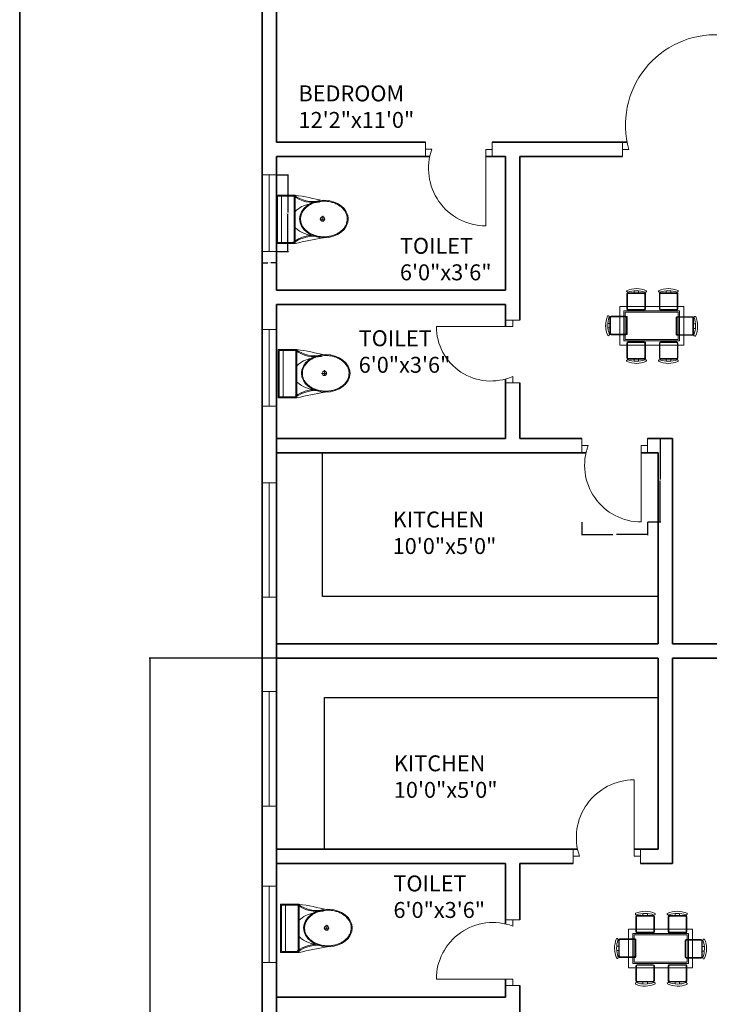
# Model space of a CAD drawing. Units: inches. Extents: x 2234 to 3001, y 1541 to 2386.
# Tile 5 of 12: x 2234 to 2450, y 1891 to 2201. Entities that reach past the tile are written whole.
import ezdxf

# ---------------------------------------------------------------- set-up
doc = ezdxf.new("R2010")
doc.units = ezdxf.units.IN
for name, color, linetype, lineweight in [('A-ANNO-DIMS', 2, 'Continuous', 18), ('A-ANNO-TTLB', 7, 'Continuous', 35), ('A-AREA-IDEN', 7, 'Continuous', 18), ('A-DOOR', 3, 'Continuous', 18), ('A-FLOR-CASE', 8, 'Continuous', 25), ('A-FLOR-FIXT', 9, 'Continuous', 18), ('A-FURN', 9, 'Continuous', 13), ('A-GLAZ', 4, 'Continuous', 18), ('A-WALL', 7, 'Continuous', 35)]:
    doc.layers.add(name, color=color, linetype=linetype, lineweight=lineweight)
doc.styles.get("Standard").update_dxf_attribs({"font": 'arial.ttf'})
doc.dimstyles.get("Standard").update_dxf_attribs({"dimtxt": 0.18, "dimasz": 0.18, "dimexe": 0.18, "dimexo": 0.0625, "dimgap": 0.09, "dimtad": 0, "dimtih": 1, "dimtoh": 1, "dimdec": 4, "dimzin": 0, "dimdsep": 46, "dimtxsty": 'Standard', "dimcen": 0.09, "dimadec": 0, "dimazin": 0, "dimtfac": 1, "dimtdec": 4, "dimtofl": 0, "dimtmove": 0, "dimatfit": 3, "dimfxl": 1, "dimtolj": 1, "dimtzin": 0, "dimarcsym": 0})

# ---------------------------------------------------------------- blocks, each defined once
blk = doc.blocks.new('A$C31115884')
for p, q in [((283, 498), (223, 498)), ((258, 466), (258, 523)), ((0, 200), (0, 0)), ((520, 200), (0, 200)), ((10, 190), (10, 10)), ((510, 190), (10, 190)), ((510, 10), (510, 190)), ((520, 0), (520, 200)), ((510, 54), (0, 54)), ((10, 10), (510, 10)), ((0, 0), (520, 0))]:
    blk.add_line(p, q)
blk.add_circle((256, 496), 23.6)
for centre, radius, start, end in [((2778, -205), 2807, 165.4549, 171.7133), ((-295, 403), 365, 324.2091, 9.3499), ((-295, 403), 375, 324.2091, 9.3499), ((806, 403), 365, 170.6501, 215.7909), ((3237, 905), 2807, 188.2867, 194.5451), ((384, 406), 293, 190.2774, 224.1564), ((139, 406), 293, 315.8436, 2.6563), ((806, 403), 375, 179.2036, 215.7909)]:
    blk.add_arc(centre, radius, start, end)
blk.add_ellipse((256, 510), major_axis=(0, -261), ratio=0.772727)
blk.add_open_spline([(256, 259), (263, 259), (270, 260), (288, 262), (299, 265), (320, 273), (330, 278), (350, 291), (360, 299), (378, 316), (386, 326), (402, 347), (409, 358), (421, 383), (427, 395), (436, 422), (440, 436), (445, 465), (447, 480), (448, 509), (448, 524), (445, 553), (443, 568), (436, 596), (432, 610), (422, 636), (416, 649), (402, 672), (395, 683), (379, 703), (370, 712), (351, 728), (341, 735), (321, 746), (310, 751), (289, 757), (278, 759), (256, 761), (245, 761), (223, 757), (212, 754), (191, 746), (181, 741), (161, 728), (151, 720), (133, 703), (125, 693), (110, 672), (103, 660), (90, 636), (85, 623), (76, 596), (72, 582), (67, 553), (66, 538), (64, 509), (65, 494), (68, 465), (70, 450), (77, 422), (81, 408), (91, 382), (97, 370), (111, 346), (118, 335), (135, 316), (144, 307), (162, 291), (172, 284), (193, 273), (203, 269), (225, 262), (236, 260), (250, 259), (253, 259), (256, 259)], degree=3, knots=[0, 0, 0, 0, 0.110105, 0.110105, 0.285049, 0.285049, 0.459994, 0.459994, 0.634938, 0.634938, 0.809882, 0.809882, 0.984827, 0.984827, 1.159771, 1.159771, 1.334715, 1.334715, 1.50966, 1.50966, 1.684604, 1.684604, 1.859549, 1.859549, 2.034493, 2.034493, 2.209437, 2.209437, 2.384382, 2.384382, 2.559326, 2.559326, 2.73427, 2.73427, 2.909215, 2.909215, 3.084159, 3.084159, 3.259103, 3.259103, 3.434048, 3.434048, 3.608992, 3.608992, 3.783936, 3.783936, 3.958881, 3.958881, 4.133825, 4.133825, 4.30877, 4.30877, 4.483714, 4.483714, 4.658658, 4.658658, 4.833603, 4.833603, 5.008547, 5.008547, 5.183491, 5.183491, 5.358436, 5.358436, 5.53338, 5.53338, 5.708324, 5.708324, 5.883269, 5.883269, 6.058213, 6.058213, 6.233158, 6.233158, 6.283185, 6.283185, 6.283185, 6.283185])
blk = doc.blocks.new('TABLE-DINING-RECT')
for points in [[(0, 12.09), (20.14, 12.09), (20.14, 0), (0, 0)], [(0, 12.09), (20.14, 12.09), (20.14, 0), (0, 0)], [(1.34, 10.74), (18.8, 10.74), (18.8, 1.34), (1.34, 1.34)], [(1.34, 10.74), (18.8, 10.74), (18.8, 1.34), (1.34, 1.34)], [(1.75, 10.34), (18.4, 10.34), (18.4, 1.75), (1.75, 1.75)], [(1.75, 10.34), (18.4, 10.34), (18.4, 1.75), (1.75, 1.75)]]:
    blk.add_lwpolyline(points, close=True)
blk = doc.blocks.new('CHAIR-DINING-A')
for points in [[(5.76, 1.34, 0.414214), (6.12, 1.7), (6.12, 6.38, 0.414214), (5.76, 6.74), (0.67, 6.74, 0.414214), (0.31, 6.38), (0.31, 1.7, 0.414214), (0.67, 1.34), (5.76, 1.34)], [(5.76, 1.34, 0.414214), (6.12, 1.7), (6.12, 6.38, 0.414214), (5.76, 6.74), (0.67, 6.74, 0.414214), (0.31, 6.38), (0.31, 1.7, 0.414214), (0.67, 1.34), (5.76, 1.34)], [(5.92, 1.12, -0.175809), (0.43, 1.16, 0.578392), (0.02, 0.71, 0.214524), (6.21, 0.62, 0.552014), (5.92, 1.12, -0.065079)], [(5.92, 1.12, -0.175809), (0.43, 1.16, 0.578392), (0.02, 0.71, 0.214524), (6.21, 0.62, 0.552014), (5.92, 1.12, -0.065079)], [(2.45, 1.34), (2.45, 0.7, -0.064759)], [(2.45, 1.34), (2.45, 0.7, -0.064759)]]:
    blk.add_lwpolyline(points, format="xyb")
blk.add_lwpolyline([(5.76, 1.5), (0.83, 1.5, -0.414214), (0.47, 1.86), (0.47, 6.22, -0.414214), (0.83, 6.58), (5.76, 6.58, -0.512069), (5.95, 6.22), (5.95, 1.86, -0.512069)], format="xyb", close=True)
blk.add_lwpolyline([(5.76, 1.5), (0.83, 1.5, -0.414214), (0.47, 1.86), (0.47, 6.22, -0.414214), (0.83, 6.58), (5.76, 6.58, -0.512069), (5.95, 6.22), (5.95, 1.86, -0.512069)], format="xyb", close=True)
blk.add_lwpolyline([(3.88, 0.69), (3.88, 1.34)])
blk.add_lwpolyline([(3.88, 0.69), (3.88, 1.34)])
blk = doc.blocks.new('CHAIR-DINING-B')
for points in [[(5.76, 1.34, 0.414214), (6.12, 1.7), (6.12, 6.38, 0.414214), (5.76, 6.74), (0.67, 6.74, 0.414214), (0.31, 6.38), (0.31, 1.7, 0.414214), (0.67, 1.34), (5.76, 1.34)], [(5.76, 1.34, 0.414214), (6.12, 1.7), (6.12, 6.38, 0.414214), (5.76, 6.74), (0.67, 6.74, 0.414214), (0.31, 6.38), (0.31, 1.7, 0.414214), (0.67, 1.34), (5.76, 1.34)], [(5.92, 1.12, -0.175809), (0.43, 1.16, 0.578392), (0.02, 0.71, 0.214524), (6.21, 0.62, 0.552014), (5.92, 1.12, -0.065079)], [(5.92, 1.12, -0.175809), (0.43, 1.16, 0.578392), (0.02, 0.71, 0.214524), (6.21, 0.62, 0.552014), (5.92, 1.12, -0.065079)], [(2.45, 1.34), (2.45, 0.7, -0.064759)], [(2.45, 1.34), (2.45, 0.7, -0.064759)]]:
    blk.add_lwpolyline(points, format="xyb")
blk.add_lwpolyline([(5.76, 1.5), (0.83, 1.5, -0.414214), (0.47, 1.86), (0.47, 6.22, -0.414214), (0.83, 6.58), (5.76, 6.58, -0.512069), (5.95, 6.22), (5.95, 1.86, -0.512069)], format="xyb", close=True)
blk.add_lwpolyline([(5.76, 1.5), (0.83, 1.5, -0.414214), (0.47, 1.86), (0.47, 6.22, -0.414214), (0.83, 6.58), (5.76, 6.58, -0.512069), (5.95, 6.22), (5.95, 1.86, -0.512069)], format="xyb", close=True)
blk.add_lwpolyline([(3.88, 0.69), (3.88, 1.34)])
blk.add_lwpolyline([(3.88, 0.69), (3.88, 1.34)])
blk = doc.blocks.new('CHAIR-DINING-C')
for points in [[(1.16, 0.43, -0.578392), (0.71, 0.02, -0.214524), (0.62, 6.21, -0.552014), (1.12, 5.92, 0.175809), (1.16, 0.43)], [(1.34, 5.76, -0.414214), (1.7, 6.11), (6.38, 6.11, -0.414214), (6.74, 5.76), (6.74, 0.66, -0.414214), (6.38, 0.31), (1.7, 0.31, -0.414214), (1.34, 0.66), (1.34, 5.76)], [(1.34, 2.45), (0.7, 2.45, 0.064759)]]:
    blk.add_lwpolyline(points, format="xyb")
blk.add_lwpolyline([(0.69, 3.88), (1.34, 3.88)])
blk.add_lwpolyline([(1.5, 5.76), (1.5, 0.83, 0.414214), (1.86, 0.47), (6.22, 0.47, 0.414214), (6.58, 0.83), (6.58, 5.76, 0.512069), (6.22, 5.95), (1.86, 5.95, 0.512069)], format="xyb", close=True)
blk = doc.blocks.new('CHAIR-DINING-D')
for points in [[(0.43, 5.57, -0.578392), (0.02, 6.03, -0.214524), (6.21, 6.11, -0.552014), (5.92, 5.62, 0.175809), (0.43, 5.57)], [(5.76, 5.4, -0.414214), (6.12, 5.04), (6.12, 0.36, -0.414214), (5.76, 0), (0.67, 0, -0.414214), (0.31, 0.36), (0.31, 5.04, -0.414214), (0.67, 5.4), (5.76, 5.4)], [(2.45, 5.4), (2.45, 6.04, 0.064759)]]:
    blk.add_lwpolyline(points, format="xyb")
blk.add_lwpolyline([(5.76, 5.24), (0.83, 5.24, 0.414214), (0.47, 4.88), (0.47, 0.52, 0.414214), (0.83, 0.16), (5.76, 0.16, 0.512069), (5.95, 0.52), (5.95, 4.88, 0.512069)], format="xyb", close=True)
blk.add_lwpolyline([(3.88, 6.05), (3.88, 5.4)])
blk = doc.blocks.new('CHAIR-DINING-F')
for points in [[(5.58, 1.34), (0.49, 1.34, -0.414214), (0.13, 1.7), (0.13, 6.38, -0.414214), (0.49, 6.74), (5.58, 6.74, -0.414214), (5.94, 6.38), (5.94, 1.7, -0.414214), (5.58, 1.34)], [(5.82, 1.16, -0.578392), (6.23, 0.71, -0.214524), (0.04, 0.62, -0.552014), (0.33, 1.12, 0.175809), (5.82, 1.16)], [(3.79, 1.34), (3.79, 0.7, 0.064759)]]:
    blk.add_lwpolyline(points, format="xyb")
blk.add_lwpolyline([(0.49, 1.5), (5.42, 1.5, 0.414214), (5.78, 1.86), (5.78, 6.22, 0.414214), (5.42, 6.58), (0.49, 6.58, 0.512069), (0.29, 6.22), (0.29, 1.86, 0.512069)], format="xyb", close=True)
blk.add_lwpolyline([(2.37, 0.69), (2.37, 1.34)])
blk = doc.blocks.new('CHAIR-DINING-G')
for points in [[(5.58, 1.34), (0.49, 1.34, -0.414214), (0.13, 1.7), (0.13, 6.38, -0.414214), (0.49, 6.74), (5.58, 6.74, -0.414214), (5.94, 6.38), (5.94, 1.7, -0.414214), (5.58, 1.34)], [(5.82, 1.16, -0.578392), (6.23, 0.71, -0.214524), (0.04, 0.62, -0.552014), (0.33, 1.12, 0.175809), (5.82, 1.16)], [(3.79, 1.34), (3.79, 0.7, 0.064759)]]:
    blk.add_lwpolyline(points, format="xyb")
blk.add_lwpolyline([(0.49, 1.5), (5.42, 1.5, 0.414214), (5.78, 1.86), (5.78, 6.22, 0.414214), (5.42, 6.58), (0.49, 6.58, 0.512069), (0.29, 6.22), (0.29, 1.86, 0.512069)], format="xyb", close=True)
blk.add_lwpolyline([(2.37, 0.69), (2.37, 1.34)])
blk = doc.blocks.new('CHAIR-DINING-H')
for points in [[(1.16, 0.43, -0.578392), (0.71, 0.02, -0.214524), (0.62, 6.21, -0.552014), (1.12, 5.92, 0.175809), (1.16, 0.43)], [(1.34, 5.76, -0.414214), (1.7, 6.11), (6.38, 6.11, -0.414214), (6.74, 5.76), (6.74, 0.66, -0.414214), (6.38, 0.31), (1.7, 0.31, -0.414214), (1.34, 0.66), (1.34, 5.76)], [(1.34, 2.45), (0.7, 2.45, 0.064759)]]:
    blk.add_lwpolyline(points, format="xyb")
blk.add_lwpolyline([(0.69, 3.88), (1.34, 3.88)])
blk.add_lwpolyline([(1.5, 5.76), (1.5, 0.83, 0.414214), (1.86, 0.47), (6.22, 0.47, 0.414214), (6.58, 0.83), (6.58, 5.76, 0.512069), (6.22, 5.95), (1.86, 5.95, 0.512069)], format="xyb", close=True)
blk = doc.blocks.new('CHAIR-DINING-I')
for points in [[(0.33, 5.62, -0.175809), (5.82, 5.57, 0.578392), (6.23, 6.03, 0.214524), (0.04, 6.11, 0.552014), (0.33, 5.62, -0.065079)], [(5.58, 5.4), (0.49, 5.4, 0.414214), (0.13, 5.04), (0.13, 0.36, 0.414214), (0.49, 0), (5.58, 0, 0.414214), (5.94, 0.36), (5.94, 5.04, 0.414214), (5.58, 5.4)], [(3.79, 5.4), (3.79, 6.04, -0.064759)]]:
    blk.add_lwpolyline(points, format="xyb")
blk.add_lwpolyline([(0.49, 5.24), (5.42, 5.24, -0.414214), (5.78, 4.88), (5.78, 0.52, -0.414214), (5.42, 0.16), (0.49, 0.16, -0.512069), (0.29, 0.52), (0.29, 4.88, -0.512069)], format="xyb", close=True)
blk.add_lwpolyline([(2.37, 6.05), (2.37, 5.4)])
blk = doc.blocks.new('WIN-24-A')
for p, q in [((0, 24), (4.5, 24)), ((4.5, 24), (2.25, 24)), ((2.25, 24), (2.25, 0)), ((2.25, 0), (0, 0)), ((0, 0), (4.5, 0))]:
    blk.add_line(p, q)
blk = doc.blocks.new('WIN-24-B')
for p, q in [((4.5, 24), (0, 24)), ((0, 24), (2.25, 24)), ((2.25, 24), (2.25, 0)), ((2.25, 0), (0, 0)), ((0, 0), (4.5, 0))]:
    blk.add_line(p, q)
blk = doc.blocks.new('WIN-36')
for p, q in [((0, 36), (4.5, 36)), ((4.5, 36), (2.25, 36)), ((2.25, 36), (2.25, 0)), ((2.25, 0), (0, 0)), ((0, 0), (4.5, 0))]:
    blk.add_line(p, q)
blk = doc.blocks.new('DOOR-SWING-24')
for p, q in [((0, 21.75), (0, 26.25)), ((0, 26.25), (0, 24)), ((20.69, 21.75), (20.69, 26.25)), ((20.69, 26.25), (20.69, 24)), ((0, 24), (2, 24)), ((20.69, 24), (18.69, 24)), ((18.69, 24), (18.69, 0))]:
    blk.add_line(p, q)
blk.add_arc((18.69, 17.81), 17.81, 159.6449, 270)
blk = doc.blocks.new('*D31')
at = {"layer": 'A-ANNO-DIMS', "color": 0, "lineweight": -2, "transparency": 16777216}
for p, q in [((2314.32, 2151.84), (2318.03, 2151.84)), ((2317.85, 2151.66), (2317.85, 2140.02)), ((2317.85, 2128.02), (2317.85, 2139.66)), ((2314.32, 2127.84), (2318.03, 2127.84))]:
    blk.add_line(p, q, dxfattribs=at)
at = {"layer": 'A-ANNO-DIMS', "color": 0, "transparency": 16777216}
for points in [[(2317.82, 2151.66), (2317.88, 2151.66), (2317.85, 2151.84)], [(2317.82, 2128.02), (2317.88, 2128.02), (2317.85, 2127.84)]]:
    blk.add_solid(points, dxfattribs=at)
at = {"layer": 'Defpoints', "color": 0, "transparency": 16777216}
for p in [(2314.25, 2151.84), (2317.85, 2151.84), (2314.25, 2127.84)]:
    blk.add_point(p, dxfattribs=at)
at = {"layer": 'A-ANNO-DIMS', "color": 0, "transparency": 16777216, "insert": (2317.85, 2139.84), "char_height": 0.18, "attachment_point": 5}
blk.add_mtext('\\A1;W-B 24 TYP.', dxfattribs=at)
blk = doc.blocks.new('*D32')
at = {"layer": 'A-ANNO-DIMS', "color": 0, "lineweight": -2, "transparency": 16777216}
for p, q in [((2309.75, 2127.77), (2309.75, 2124.06)), ((2314.25, 2127.77), (2314.25, 2124.06)), ((2309.93, 2124.24), (2311.55, 2124.24)), ((2314.07, 2124.24), (2312.46, 2124.24))]:
    blk.add_line(p, q, dxfattribs=at)
at = {"layer": 'A-ANNO-DIMS', "color": 0, "transparency": 16777216}
for points in [[(2309.93, 2124.27), (2309.93, 2124.21), (2309.75, 2124.24)], [(2314.07, 2124.27), (2314.07, 2124.21), (2314.25, 2124.24)]]:
    blk.add_solid(points, dxfattribs=at)
at = {"layer": 'Defpoints', "color": 0, "transparency": 16777216}
for p in [(2309.75, 2127.84), (2314.25, 2127.84), (2314.25, 2124.24)]:
    blk.add_point(p, dxfattribs=at)
at = {"layer": 'A-ANNO-DIMS', "color": 0, "transparency": 16777216, "insert": (2312, 2124.24), "char_height": 0.18, "attachment_point": 5}
blk.add_mtext('\\A1;5 TYP.', dxfattribs=at)
blk = doc.blocks.new('*D59')
at = {"layer": 'A-ANNO-DIMS', "color": 0, "lineweight": -2, "transparency": 16777216}
for p, q in [((2430.98, 2069.11), (2435.04, 2069.11)), ((2434.86, 2068.93), (2434.86, 2056.17)), ((2434.86, 2043.04), (2434.86, 2055.8)), ((2430.98, 2042.86), (2435.04, 2042.86))]:
    blk.add_line(p, q, dxfattribs=at)
at = {"layer": 'A-ANNO-DIMS', "color": 0, "transparency": 16777216}
for points in [[(2434.83, 2068.93), (2434.89, 2068.93), (2434.86, 2069.11)], [(2434.83, 2043.04), (2434.89, 2043.04), (2434.86, 2042.86)]]:
    blk.add_solid(points, dxfattribs=at)
at = {"layer": 'Defpoints', "color": 0, "transparency": 16777216}
for p in [(2430.92, 2069.11), (2434.86, 2069.11), (2430.92, 2042.86)]:
    blk.add_point(p, dxfattribs=at)
at = {"layer": 'A-ANNO-DIMS', "color": 0, "transparency": 16777216, "insert": (2434.86, 2055.99), "char_height": 0.18, "attachment_point": 5}
blk.add_mtext('\\A1;DOOR 26 TYP.', dxfattribs=at)
blk = doc.blocks.new('*D60')
at = {"layer": 'A-ANNO-DIMS', "color": 0, "lineweight": -2, "transparency": 16777216}
for p, q in [((2410.2, 2042.8), (2410.2, 2038.74)), ((2430.92, 2042.8), (2430.92, 2038.74)), ((2410.38, 2038.92), (2420.03, 2038.92)), ((2430.74, 2038.92), (2421.09, 2038.92))]:
    blk.add_line(p, q, dxfattribs=at)
at = {"layer": 'A-ANNO-DIMS', "color": 0, "transparency": 16777216}
for points in [[(2410.38, 2038.95), (2410.38, 2038.89), (2410.2, 2038.92)], [(2430.74, 2038.95), (2430.74, 2038.89), (2430.92, 2038.92)]]:
    blk.add_solid(points, dxfattribs=at)
at = {"layer": 'Defpoints', "color": 0, "transparency": 16777216}
for p in [(2410.2, 2042.86), (2430.92, 2042.86), (2430.92, 2038.92)]:
    blk.add_point(p, dxfattribs=at)
at = {"layer": 'A-ANNO-DIMS', "color": 0, "transparency": 16777216, "insert": (2420.56, 2038.92), "char_height": 0.18, "attachment_point": 5}
blk.add_mtext('\\A1;21 TYP.', dxfattribs=at)
blk = doc.blocks.new('*D63')
at = {"layer": 'A-ANNO-DIMS', "color": 0, "lineweight": -2, "transparency": 16777216}
for p, q in [((2314.19, 2000.11), (2274.22, 2000.11)), ((2274.4, 1999.93), (2274.4, 1851.29)), ((2274.4, 1702.29), (2274.4, 1850.93)), ((2309.69, 1702.11), (2274.22, 1702.11))]:
    blk.add_line(p, q, dxfattribs=at)
at = {"layer": 'A-ANNO-DIMS', "color": 0, "transparency": 16777216}
for points in [[(2274.37, 1999.93), (2274.43, 1999.93), (2274.4, 2000.11)], [(2274.37, 1702.29), (2274.43, 1702.29), (2274.4, 1702.11)]]:
    blk.add_solid(points, dxfattribs=at)
at = {"layer": 'Defpoints', "color": 0, "transparency": 16777216}
for p in [(2274.4, 2000.11), (2314.25, 2000.11), (2309.75, 1702.11)]:
    blk.add_point(p, dxfattribs=at)
at = {"layer": 'A-ANNO-DIMS', "color": 0, "transparency": 16777216, "insert": (2274.4, 1851.11), "char_height": 0.18, "attachment_point": 5}
blk.add_mtext('\\A1;298', dxfattribs=at)

msp = doc.modelspace()

# ---------------------------------------------------------------- linework, layer by layer
at = {"layer": 'A-ANNO-TTLB'}
msp.add_lwpolyline([(2233.5367, 2385.7012), (3001.3383, 2385.7012), (3001.3383, 1541.435), (2233.5367, 1541.435)], close=True, dxfattribs=at)
at = {"layer": 'A-DOOR'}
for p, q in [((2361.0969, 2161.6071), (2361.0969, 2162.111)), ((2361.0969, 2162.111), (2361.0969, 2159.9395)), ((2382.0512, 2157.611), (2382.0512, 2162.111)), ((2382.0512, 2162.111), (2382.0512, 2159.861)), ((2423.0287, 2162.111), (2423.0287, 2157.611)), ((2361.0969, 2157.611), (2361.0969, 2161.6071)), ((2361.0969, 2159.9395), (2363.0969, 2159.9395)), ((2382.0512, 2159.861), (2380.0512, 2159.861)), ((2380.0512, 2159.861), (2380.0512, 2135.861)), ((2423.0287, 2157.611), (2423.0287, 2159.861)), ((2423.0287, 2159.861), (2425.0287, 2159.861)), ((2386.2534, 2106.2721), (2390.7534, 2106.2721)), ((2390.7534, 2106.2721), (2388.5034, 2106.2721)), ((2388.5034, 2106.2721), (2388.5034, 2104.2721)), ((2388.5034, 2104.2721), (2364.5034, 2104.2721)), ((2388.5034, 2086.5533), (2388.5034, 2088.5533)), ((2386.2534, 2086.5533), (2390.7534, 2086.5533)), ((2390.7534, 2086.5533), (2388.5034, 2086.5533)), ((2426.6497, 1937.861), (2426.6497, 1961.861)), ((2407.4857, 1940.111), (2407.4857, 1935.611)), ((2428.6497, 1940.111), (2428.6497, 1935.611)), ((2407.4857, 1935.611), (2407.4857, 1937.861)), ((2407.4857, 1937.861), (2409.4857, 1937.861)), ((2428.6497, 1937.861), (2426.6497, 1937.861)), ((2428.6497, 1935.611), (2428.6497, 1937.861))]:
    msp.add_line(p, q, dxfattribs=at)
for centre, radius, start, end in [((2452.2624, 2167.5859), 28.3081, 87.231325, 195.836074), ((2380.0512, 2153.8692), 18.0082, 160.300833, 270), ((2381.651, 2104.2721), 17.1475, 180, 293.554455), ((2426.6497, 1943.7235), 18.1376, 90, 198.857849)]:
    msp.add_arc(centre, radius, start, end, dxfattribs=at)
at = {"layer": 'A-FLOR-CASE'}
for p, q in [((2328.7508, 2019.4407), (2328.7508, 2064.611)), ((2434.2534, 2019.4407), (2328.7508, 2019.4407)), ((2329.3733, 1940.111), (2329.3733, 1987.7196)), ((2329.3733, 1987.7196), (2434.2534, 1987.7196))]:
    msp.add_line(p, q, dxfattribs=at)
at = {"layer": 'A-FURN'}
for points in [[(2424.6306, 2115.0385, -0.17580919), (2430.1173, 2114.9969, 0.57839206), (2430.5329, 2115.454, 0.21452438), (2424.3397, 2115.5371, 0.55201397), (2424.6306, 2115.0385, -0.06507904)], [(2428.0954, 2114.8183), (2428.0954, 2115.4624, -0.06475861)], [(2429.8845, 2114.8183), (2424.7909, 2114.8183, 0.41421356), (2424.4345, 2114.4619), (2424.4345, 2109.7784, 0.41421356), (2424.7909, 2109.4221), (2429.8845, 2109.4221, 0.41421356), (2430.2408, 2109.7784), (2430.2408, 2114.4619, 0.41421356), (2429.8845, 2114.8183)], [(2418.8906, 2101.7889, -0.57839206), (2418.4335, 2101.3732, -0.21452438), (2418.3504, 2107.5665, -0.55201397), (2418.849, 2107.2755, 0.17580937), (2418.8906, 2101.7889)], [(2419.0692, 2107.1152, -0.41421356), (2419.4256, 2107.4716), (2424.1091, 2107.4716, -0.41421356), (2424.4654, 2107.1152), (2424.4654, 2102.0216, -0.41421356), (2424.1091, 2101.6653), (2419.4256, 2101.6653, -0.41421356), (2419.0692, 2102.0216), (2419.0692, 2107.1152)], [(2419.0692, 2103.8108), (2418.425, 2103.8108, 0.06475861)], [(2440.0627, 2093.9991, 0.41421356), (2440.419, 2094.3554), (2440.419, 2099.0389, 0.41421356), (2440.0627, 2099.3953), (2434.9691, 2099.3953, 0.41421356), (2434.6127, 2099.0389), (2434.6127, 2094.3554, 0.41421356), (2434.9691, 2093.9991), (2440.0627, 2093.9991)], [(2440.0627, 2093.9989, 0.41421356), (2440.4191, 2094.3552), (2440.4191, 2099.0387, 0.41421356), (2440.0627, 2099.395), (2434.9691, 2099.395, 0.41421356), (2434.6127, 2099.0387), (2434.6127, 2094.3552, 0.41421356), (2434.9691, 2093.9989), (2440.0627, 2093.9989)], [(2440.2229, 2093.7789, -0.17580928), (2434.7363, 2093.8204, 0.57839206), (2434.3207, 2093.3634, 0.21452438), (2440.5139, 2093.2803, 0.55201397), (2440.2229, 2093.7789, -0.06507904)], [(2440.223, 2093.7787, -0.17580928), (2434.7363, 2093.8202, 0.57839206), (2434.3207, 2093.3632, 0.21452438), (2440.5139, 2093.2801, 0.55201397), (2440.223, 2093.7787, -0.06507904)], [(2436.7582, 2093.9991), (2436.7582, 2093.3549, -0.06475861)], [(2436.7582, 2093.9989), (2436.7582, 2093.3547, -0.06475861)], [(2427.4218, 1919.4504, -0.17580919), (2432.9085, 1919.4088, 0.57839206), (2433.3241, 1919.8659, 0.21452438), (2427.1309, 1919.949, 0.55201397), (2427.4218, 1919.4504, -0.06507904)], [(2427.4218, 1919.4501, -0.17580919), (2432.9085, 1919.4086, 0.57839206), (2433.3241, 1919.8656, 0.21452438), (2427.1309, 1919.9487, 0.55201397), (2427.4218, 1919.4501, -0.06507904)], [(2437.5275, 1919.4088, -0.57839206), (2437.1118, 1919.8659, -0.21452438), (2443.3051, 1919.949, -0.55201397), (2443.0141, 1919.4504, 0.1758092), (2437.5275, 1919.4088)], [(2432.6757, 1919.2301), (2427.5821, 1919.2301, 0.41421356), (2427.2257, 1918.8738), (2427.2257, 1914.1903, 0.41421356), (2427.5821, 1913.834), (2432.6757, 1913.834, 0.41421356), (2433.032, 1914.1903), (2433.032, 1918.8738, 0.41421356), (2432.6757, 1919.2301)], [(2432.6757, 1919.2299), (2427.5821, 1919.2299, 0.41421356), (2427.2257, 1918.8736), (2427.2257, 1914.1901, 0.41421356), (2427.5821, 1913.8338), (2432.6757, 1913.8338, 0.41421356), (2433.032, 1914.1901), (2433.032, 1918.8736, 0.41421356), (2432.6757, 1919.2299)], [(2430.8865, 1919.2301), (2430.8865, 1919.8743, -0.06475861)], [(2430.8866, 1919.2299), (2430.8866, 1919.8741, -0.06475861)], [(2442.8539, 1919.2301, -0.41421356), (2443.2102, 1918.8738), (2443.2102, 1914.1903, -0.41421356), (2442.8539, 1913.834), (2437.7603, 1913.834, -0.41421356), (2437.4039, 1914.1903), (2437.4039, 1918.8738, -0.41421356), (2437.7603, 1919.2301), (2442.8539, 1919.2301)], [(2439.5494, 1919.2301), (2439.5494, 1919.8743, 0.06475861)], [(2421.6817, 1906.201, -0.57839206), (2421.2247, 1905.7853, -0.21452438), (2421.1416, 1911.9786, -0.55201397), (2421.6402, 1911.6876, 0.17580937), (2421.6817, 1906.201)], [(2421.8604, 1911.5273, -0.41421356), (2422.2168, 1911.8837), (2426.9002, 1911.8837, -0.41421356), (2427.2566, 1911.5273), (2427.2566, 1906.4337, -0.41421356), (2426.9002, 1906.0774), (2422.2168, 1906.0774, -0.41421356), (2421.8604, 1906.4337), (2421.8604, 1911.5273)], [(2448.0901, 1911.3529, 0.41421356), (2447.7337, 1911.7093), (2443.0503, 1911.7093, 0.41421356), (2442.6939, 1911.3529), (2442.6939, 1906.2593, 0.41421356), (2443.0503, 1905.9029), (2447.7337, 1905.9029, 0.41421356), (2448.0901, 1906.2593), (2448.0901, 1911.3529)], [(2448.0901, 1911.3527, 0.41421356), (2447.7338, 1911.709), (2443.0503, 1911.709, 0.41421356), (2442.6939, 1911.3527), (2442.6939, 1906.2591, 0.41421356), (2443.0503, 1905.9027), (2447.7338, 1905.9027, 0.41421356), (2448.0901, 1906.2591), (2448.0901, 1911.3527)], [(2448.3103, 1911.5132, -0.17580919), (2448.2688, 1906.0265, 0.57839206), (2448.7258, 1905.6109, 0.21452438), (2448.8089, 1911.8041, 0.55201397), (2448.3103, 1911.5132, -0.06507904)], [(2448.3103, 1911.5129, -0.17580919), (2448.2688, 1906.0263, 0.57839206), (2448.7258, 1905.6107, 0.21452438), (2448.8089, 1911.8039, 0.55201397), (2448.3103, 1911.5129, -0.06507904)], [(2421.8604, 1908.2229), (2421.2162, 1908.2229, 0.06475861)], [(2448.0901, 1908.0484), (2448.7343, 1908.0484, -0.06475861)], [(2448.0901, 1908.0482), (2448.7343, 1908.0482, -0.06475861)], [(2432.6757, 1898.411), (2427.5821, 1898.411, -0.41421356), (2427.2257, 1898.7673), (2427.2257, 1903.4508, -0.41421356), (2427.5821, 1903.8071), (2432.6757, 1903.8071, -0.41421356), (2433.032, 1903.4508), (2433.032, 1898.7673, -0.41421356), (2432.6757, 1898.411)], [(2432.6757, 1898.4108), (2427.5821, 1898.4108, -0.41421356), (2427.2257, 1898.7671), (2427.2257, 1903.4506, -0.41421356), (2427.5821, 1903.8069), (2432.6757, 1903.8069, -0.41421356), (2433.032, 1903.4506), (2433.032, 1898.7671, -0.41421356), (2432.6757, 1898.4108)], [(2432.9085, 1898.2323, -0.57839206), (2433.3241, 1897.7753, -0.21452438), (2427.1309, 1897.6922, -0.55201397), (2427.4218, 1898.1908, 0.17580929), (2432.9085, 1898.2323)], [(2432.9085, 1898.2321, -0.57839206), (2433.3241, 1897.775, -0.21452438), (2427.1309, 1897.6919, -0.55201397), (2427.4218, 1898.1905, 0.17580929), (2432.9085, 1898.2321)], [(2430.8865, 1898.411), (2430.8865, 1897.7668, 0.06475861)], [(2430.8866, 1898.4108), (2430.8866, 1897.7666, 0.06475861)]]:
    msp.add_lwpolyline(points, format="xyb", dxfattribs=at)
for points in [[(2426.6696, 2115.4742), (2426.6696, 2114.8183)], [(2418.4133, 2105.2365), (2419.0692, 2105.2365)], [(2438.184, 2093.3432), (2438.184, 2093.9991)], [(2438.184, 2093.343), (2438.184, 2093.9989)], [(2429.4608, 1919.886), (2429.4608, 1919.2301)], [(2429.4608, 1919.8858), (2429.4608, 1919.2299)], [(2440.9752, 1919.886), (2440.9752, 1919.2301)], [(2421.2045, 1909.6486), (2421.8604, 1909.6486)], [(2448.746, 1909.4742), (2448.0901, 1909.4742)], [(2448.746, 1909.474), (2448.0901, 1909.474)], [(2429.4608, 1897.7551), (2429.4608, 1898.411)], [(2429.4608, 1897.7549), (2429.4608, 1898.4108)]]:
    msp.add_lwpolyline(points, dxfattribs=at)
for points in [[(2424.7931, 2114.6577), (2429.724, 2114.6577, -0.41421356), (2430.0803, 2114.3014), (2430.0803, 2109.939, -0.41421356), (2429.724, 2109.5826), (2424.7931, 2109.5826, -0.51206948), (2424.5951, 2109.939), (2424.5951, 2114.3014, -0.51206948)], [(2419.2298, 2107.1131), (2419.2298, 2102.1822, 0.41421356), (2419.5861, 2101.8258), (2423.9485, 2101.8258, 0.41421356), (2424.3049, 2102.1822), (2424.3049, 2107.1131, 0.51206948), (2423.9485, 2107.3111), (2419.5861, 2107.3111, 0.51206948)], [(2440.0605, 2094.1596), (2435.1296, 2094.1596, -0.41421356), (2434.7733, 2094.516), (2434.7733, 2098.8784, -0.41421356), (2435.1296, 2099.2347), (2440.0605, 2099.2347, -0.51206948), (2440.2585, 2098.8784), (2440.2585, 2094.516, -0.51206948)], [(2440.0605, 2094.1594), (2435.1296, 2094.1594, -0.41421356), (2434.7733, 2094.5158), (2434.7733, 2098.8782, -0.41421356), (2435.1296, 2099.2345), (2440.0605, 2099.2345, -0.51206948), (2440.2585, 2098.8782), (2440.2585, 2094.5158, -0.51206948)], [(2427.5842, 1919.0696), (2432.5151, 1919.0696, -0.41421356), (2432.8715, 1918.7133), (2432.8715, 1914.3509, -0.41421356), (2432.5151, 1913.9945), (2427.5842, 1913.9945, -0.51206948), (2427.3863, 1914.3509), (2427.3863, 1918.7133, -0.51206948)], [(2427.5842, 1919.0694), (2432.5151, 1919.0694, -0.41421356), (2432.8715, 1918.713), (2432.8715, 1914.3506, -0.41421356), (2432.5151, 1913.9943), (2427.5842, 1913.9943, -0.51206948), (2427.3863, 1914.3506), (2427.3863, 1918.713, -0.51206948)], [(2442.8517, 1919.0696), (2437.9208, 1919.0696, 0.41421356), (2437.5645, 1918.7133), (2437.5645, 1914.3509, 0.41421356), (2437.9208, 1913.9945), (2442.8517, 1913.9945, 0.51206948), (2443.0497, 1914.3509), (2443.0497, 1918.7133, 0.51206948)], [(2422.0209, 1911.5252), (2422.0209, 1906.5943, 0.41421356), (2422.3773, 1906.2379), (2426.7397, 1906.2379, 0.41421356), (2427.096, 1906.5943), (2427.096, 1911.5252, 0.51206948), (2426.7397, 1911.7232), (2422.3773, 1911.7232, 0.51206948)], [(2447.9296, 1911.3507), (2447.9296, 1906.4198, -0.41421356), (2447.5732, 1906.0635), (2443.2108, 1906.0635, -0.41421356), (2442.8545, 1906.4198), (2442.8545, 1911.3507, -0.51206948), (2443.2108, 1911.5487), (2447.5732, 1911.5487, -0.51206948)], [(2447.9296, 1911.3505), (2447.9296, 1906.4196, -0.41421356), (2447.5732, 1906.0633), (2443.2108, 1906.0633, -0.41421356), (2442.8545, 1906.4196), (2442.8545, 1911.3505, -0.51206948), (2443.2108, 1911.5485), (2447.5732, 1911.5485, -0.51206948)], [(2427.5842, 1898.5715), (2432.5151, 1898.5715, 0.41421356), (2432.8715, 1898.9279), (2432.8715, 1903.2903, 0.41421356), (2432.5151, 1903.6466), (2427.5842, 1903.6466, 0.51206948), (2427.3863, 1903.2903), (2427.3863, 1898.9279, 0.51206948)], [(2427.5842, 1898.5713), (2432.5151, 1898.5713, 0.41421356), (2432.8715, 1898.9276), (2432.8715, 1903.29, 0.41421356), (2432.5151, 1903.6464), (2427.5842, 1903.6464, 0.51206948), (2427.3863, 1903.29), (2427.3863, 1898.9276, 0.51206948)]]:
    msp.add_lwpolyline(points, format="xyb", close=True, dxfattribs=at)
at = {"layer": 'A-GLAZ'}
for p, q in [((2314.2534, 1989.5826), (2309.7534, 1989.5826)), ((2309.7534, 1989.5826), (2312.0034, 1989.5826)), ((2312.0034, 1989.5826), (2312.0034, 1953.5826)), ((2312.0034, 1953.5826), (2309.7534, 1953.5826)), ((2309.7534, 1953.5826), (2314.2534, 1953.5826))]:
    msp.add_line(p, q, dxfattribs=at)
at = {"layer": 'A-WALL'}
for p, q in [((2309.7534, 2298.611), (2309.7534, 1702.111)), ((2314.2534, 2294.111), (2314.2534, 2162.111)), ((2314.2534, 2162.111), (2361.0969, 2162.111)), ((2382.0512, 2162.111), (2424.4888, 2162.111)), ((2386.2534, 2162.111), (2390.7534, 2162.111)), ((2314.2534, 2157.611), (2362.436, 2157.611)), ((2314.2534, 2157.611), (2314.2534, 2115.611)), ((2380.0512, 2157.611), (2386.2534, 2157.611)), ((2386.2534, 2115.611), (2386.2534, 2157.611)), ((2390.7534, 2157.611), (2390.7534, 2106.2721)), ((2390.7534, 2157.611), (2423.0287, 2157.611)), ((2314.2534, 2115.611), (2386.2534, 2115.611)), ((2314.2534, 2111.111), (2386.2534, 2111.111)), ((2314.2534, 2111.111), (2314.2534, 2069.111)), ((2386.2534, 2104.2721), (2386.2534, 2111.111)), ((2386.2534, 2069.111), (2386.2534, 2087.7538)), ((2390.7534, 2086.5533), (2390.7534, 2069.111)), ((2314.2534, 2069.111), (2386.2534, 2069.111)), ((2314.2534, 2069.111), (2314.2534, 1706.611)), ((2390.7534, 2069.111), (2410.2281, 2069.111)), ((2430.9225, 2069.111), (2438.7534, 2069.111)), ((2438.7534, 2069.111), (2438.7534, 2064.611)), ((2314.2534, 2064.611), (2390.7534, 2064.611)), ((2314.2534, 2064.611), (2386.2534, 2064.611)), ((2411.5584, 2064.611), (2390.7534, 2064.611)), ((2434.2534, 2064.611), (2428.9225, 2064.611)), ((2434.2534, 2064.611), (2434.2534, 2004.611)), ((2438.7534, 2064.611), (2438.7534, 2004.611)), ((2314.2534, 2004.611), (2434.2534, 2004.611)), ((2438.7534, 2004.611), (2560.3722, 2004.611)), ((2314.2534, 2000.111), (2434.2534, 2000.111)), ((2434.2534, 2000.111), (2434.2534, 1940.111)), ((2438.7534, 2000.111), (2558.623, 2000.111)), ((2438.7534, 2000.111), (2438.7534, 1935.611)), ((2314.2534, 1940.111), (2408.8755, 1940.111)), ((2426.6497, 1940.111), (2434.2534, 1940.111)), ((2314.2534, 1935.611), (2386.2534, 1935.611)), ((2386.2534, 1916.599), (2386.2534, 1935.611)), ((2390.7534, 1935.611), (2390.7534, 1917.9293)), ((2390.7534, 1935.611), (2407.4857, 1935.611)), ((2428.6497, 1935.611), (2438.7534, 1935.611)), ((2386.2534, 1893.611), (2386.2534, 1899.2352)), ((2390.7534, 1897.2352), (2390.7534, 1872.7928)), ((2314.2534, 1893.611), (2386.2534, 1893.611)), ((2314.2534, 1893.611), (2386.2534, 1893.611))]:
    msp.add_line(p, q, dxfattribs=at)

# ---------------------------------------------------------------- block references
at = {"layer": 'A-DOOR'}
msp.add_blockref('DOOR-SWING-24', (2410.228, 2042.861), dxfattribs=at)
at = {"layer": 'A-DOOR', "rotation": 270}
msp.add_blockref('DOOR-SWING-24', (2364.5034, 1917.9296), dxfattribs=at)
at = {"layer": 'A-FLOR-FIXT', "xscale": 0.0292470664339069, "yscale": 0.0292470664339069, "zscale": 0.0292470664339069, "rotation": 270}
for p in [(2314.2534, 2145.5024), (2314.8221, 2097.0313), (2315.4982, 1922.8215)]:
    msp.add_blockref('A$C31115884', p, dxfattribs=at)
at = {"layer": 'A-FURN'}
for name, p in [('CHAIR-DINING-I', (2424.301, 2109.422)), ('CHAIR-DINING-D', (2434.304, 2109.4222)), ('CHAIR-DINING-D', (2434.304, 2109.422)), ('TABLE-DINING-RECT', (2422.1388, 2098.4301)), ('CHAIR-DINING-H', (2417.728, 2101.357)), ('CHAIR-DINING-G', (2424.301, 2092.658)), ('CHAIR-DINING-F', (2424.3009, 2092.6578)), ('CHAIR-DINING-D', (2437.0952, 1913.8339)), ('TABLE-DINING-RECT', (2424.93, 1902.842)), ('CHAIR-DINING-C', (2420.5191, 1905.7689)), ('CHAIR-DINING-A', (2437.095, 1897.069))]:
    msp.add_blockref(name, p, dxfattribs=at)
at = {"layer": 'A-FURN', "rotation": 90}
msp.add_blockref('CHAIR-DINING-B', (2446.6409, 2101.1821), dxfattribs=at)
at = {"layer": 'A-GLAZ'}
for name, p in [('WIN-24-B', (2309.753, 2127.836)), ('WIN-24-B', (2309.753, 2079.2707)), ('WIN-36', (2309.753, 2019.197))]:
    msp.add_blockref(name, p, dxfattribs=at)
at = {"layer": 'A-GLAZ', "rotation": 180}
msp.add_blockref('WIN-24-A', (2314.2539, 1928.4846), dxfattribs=at)

# ---------------------------------------------------------------- texts
at = {"layer": 'A-AREA-IDEN', "char_height": 5, "attachment_point": 1}
for s, width, insert in [('BEDROOM\\P12\'2"x11\'0"', 107.50727, (2321.1878, 2179.9667)), ('TOILET\\P6\'0"x3\'6"', 90.530785, (2353.0593, 2132.0967)), ('TOILET\\P6\'0"x3\'6"', 77.210486, (2340.0949, 2103.0548)), ('KITCHEN\\P10\'0"x5\'0"', 151.830771, (2350.7824, 2046.1244)), ('KITCHEN\\P10\'0"x5\'0"', 120.351356, (2351.1504, 1969.5466)), ('TOILET\\P6\'0"x3\'6"', 74.887127, (2351.0219, 1931.8266))]:
    msp.add_mtext_dynamic_manual_height_columns(s, width=width, gutter_width=12.5, heights=[0], dxfattribs=dict(at, insert=insert))

# ---------------------------------------------------------------- dimensions: what is measured, and where the dimension line sits
at = {"layer": 'A-ANNO-DIMS'}
for base, p1, p2, text, picture, middle in [((2317.8534, 2151.836), (2314.2534, 2127.836), (2314.2534, 2151.836), 'W-B <> TYP.', '*D31', (2317.8534, 2139.836)), ((2434.86, 2069.111), (2430.9225, 2042.861), (2430.9225, 2069.111), 'DOOR <> TYP.', '*D59', (2434.86, 2055.986))]:
    dim = msp.add_linear_dim(base=base, p1=p1, p2=p2, angle=90, text=text, dimstyle='Standard', override={"dimdec": 0, "dimlfac": 1, "dimrnd": 0, "dimzin": 0, "dimdsep": 46, "dimlunit": 2}, dxfattribs=at)
    dim.commit()
    dim.dimension.update_dxf_attribs({"geometry": picture, "text_midpoint": middle})
for base, p1, p2, picture, middle in [((2314.2534479174, 2124.2360341269), (2309.7534479174, 2127.8360341269), (2314.2534479174, 2127.8360341269), '*D32', (2312.0034479174, 2124.2360341269)), ((2430.9225, 2038.9235), (2410.2005, 2042.861), (2430.9225, 2042.861), '*D60', (2420.5615, 2038.9235))]:
    dim = msp.add_linear_dim(base=base, p1=p1, p2=p2, text='<> TYP.', dimstyle='Standard', override={"dimdec": 0, "dimlfac": 1, "dimrnd": 0, "dimzin": 0, "dimdsep": 46, "dimlunit": 2}, dxfattribs=at)
    dim.commit()
    dim.dimension.update_dxf_attribs({"geometry": picture, "text_midpoint": middle})
dim = msp.add_linear_dim(base=(2274.4034, 2000.111), p1=(2309.7534, 1702.111), p2=(2314.2534, 2000.111), angle=90, dimstyle='Standard', override={"dimdec": 0, "dimlfac": 1, "dimrnd": 0, "dimzin": 0, "dimdsep": 46, "dimlunit": 2}, dxfattribs=at)
dim.commit()
dim.dimension.update_dxf_attribs({"geometry": '*D63', "text_midpoint": (2274.4034, 1851.111)})

doc.saveas('drawing.dxf')
